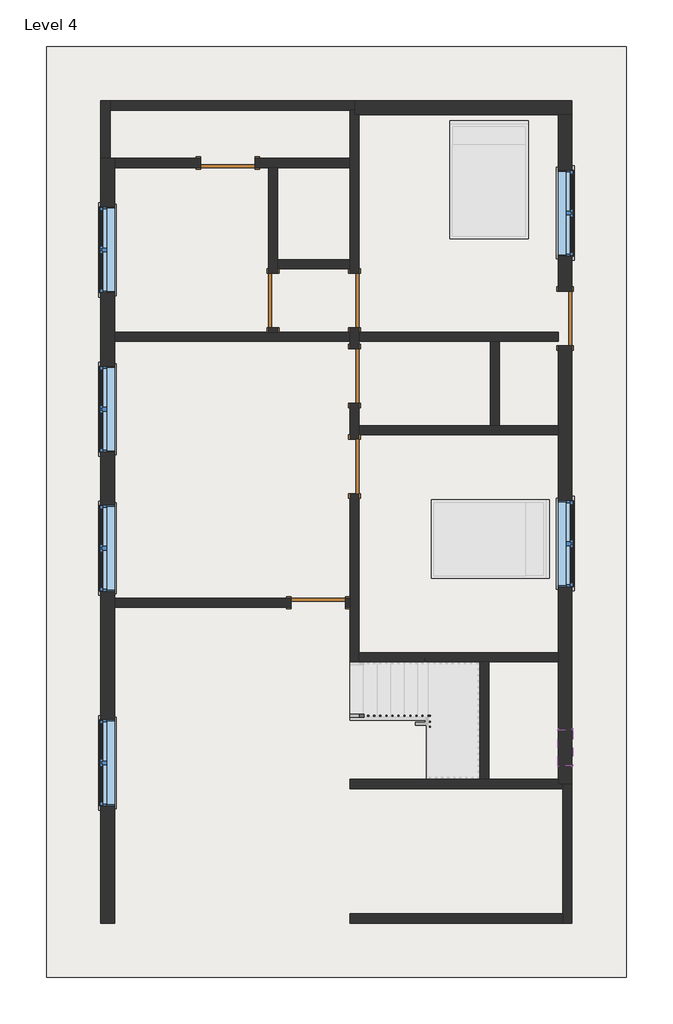
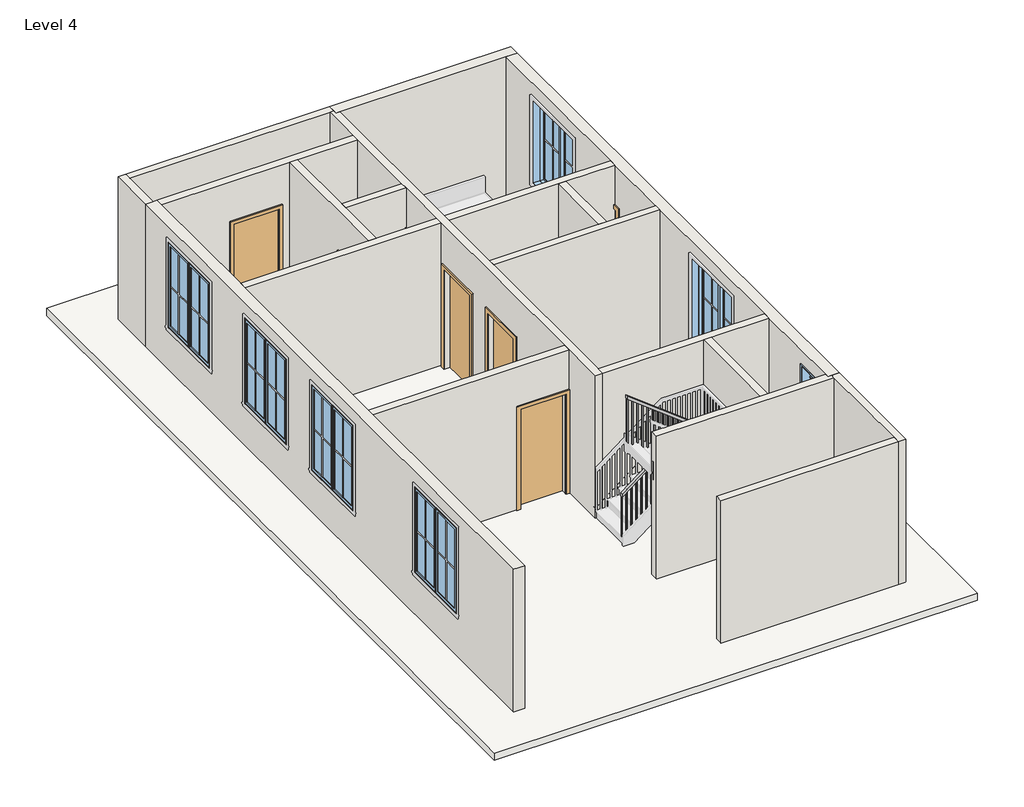
# One storey, part 1 of 2: 18 walls, 7 doors, 7 windows, 1 railing, 1 roof.
"""IFC4 building model written with IfcOpenShell, lengths in millimetres."""

from ifc_helpers import new_model, si_unit, frame, origin, place, context, project, spatial, polyline, outline, extrude, faceted_brep, transform, mapped, element, save
from components import door_686f89d2, door_16372e1c, door_0ca8825f, window_9ac97e1a, window_f2d8fef0

model = new_model("IFC4")

# Units and contexts
model_context = context("Model", 3, world=origin())
ifc_project = project(units=[si_unit("LENGTHUNIT", "METRE", prefix="MILLI")], contexts=[model_context])

# Site, building, storey
site = spatial("IfcSite", under=ifc_project)
building = spatial("IfcBuilding", under=site)
storey = spatial("IfcBuildingStorey", under=building, Name="Level 4", Elevation=6400.8)

# Doors
placement = place(None, origin())
door_shape = door_686f89d2(model_context)
element("IfcDoor", 1, ObjectType="Single-Flush : 36\" x 84\"", at=placement, inside=storey, context=model_context, shape_type="MappedRepresentation", body=[
    mapped(door_shape, transform((-2318.0415352, 3143.9226491, 6400.8), x_axis=(0.0, -1.0, 0.0), y_axis=(1.0, 0.0, 0.0), z_axis=(0.0, 0.0, 1.0))),
])
element("IfcDoor", 2, ObjectType="Single-Flush : 36\" x 84\"", at=placement, inside=storey, context=model_context, shape_type="MappedRepresentation", body=[
    mapped(door_shape, transform((-946.4415352, 3143.7222669, 6400.8), x_axis=(0.0, 1.0, 0.0), y_axis=(-1.0, 0.0, 0.0), z_axis=(0.0, 0.0, 1.0))),
])
element("IfcDoor", 3, ObjectType="Single-Flush : 36\" x 84\"", at=placement, inside=storey, context=model_context, shape_type="MappedRepresentation", body=[
    mapped(door_shape, transform((-946.4415352, 1874.1230313, 6400.8), x_axis=(0.0, 1.0, 0.0), y_axis=(-1.0, 0.0, 0.0), z_axis=(0.0, 0.0, 1.0))),
])
element("IfcDoor", 4, ObjectType="Single-Flush : 36\" x 84\"", at=placement, inside=storey, context=model_context, shape_type="MappedRepresentation", body=[
    mapped(door_shape, transform((-946.4415352, 350.1230313, 6400.8), x_axis=(0.0, 1.0, 0.0), y_axis=(-1.0, 0.0, 0.0), z_axis=(0.0, 0.0, 1.0))),
])
element("IfcDoor", 5, ObjectType="Single-Flush : 36\" x 84\"", at=placement, inside=storey, context=model_context, shape_type="MappedRepresentation", body=[
    mapped(door_shape, transform((-3080.0415352, 5453.9645078, 6400.8), x_axis=(1.0, 0.0, 0.0), y_axis=(0.0, 1.0, 0.0), z_axis=(0.0, 0.0, 1.0))),
])
door_2_shape = door_16372e1c(model_context)
element("IfcDoor", 6, ObjectType="Single-Flush : 36\" x 84\"", at=placement, inside=storey, context=model_context, shape_type="MappedRepresentation", body=[
    mapped(door_2_shape, transform((-1556.0415352, -1935.8769687, 6400.8), x_axis=(1.0, 0.0, 0.0), y_axis=(0.0, 1.0, 0.0), z_axis=(0.0, 0.0, 1.0))),
])
door_3_shape = door_0ca8825f(model_context)
element("IfcDoor", 7, ObjectType="Single-Flush : 36\" x 84\"", at=placement, inside=storey, context=model_context, shape_type="MappedRepresentation", body=[
    mapped(door_3_shape, transform((2596.8584648, 2839.3230313, 6400.8), x_axis=(0.0, -1.0, 0.0), y_axis=(1.0, 0.0, 0.0), z_axis=(0.0, 0.0, 1.0))),
])

# Railing
element("IfcRailing", 8, ObjectType="Handrail - Rectangular", at=placement, inside=storey, context=model_context, shape_type="SolidModel", body=[
    faceted_brep([(-1022.6415352, -3810.4539367, 7484.5333333), (-1022.6415352, -3810.4539367, 7420.3783974), (-1022.6415352, -3861.2539367, 7420.3783974), (-1022.6415352, -3861.2539367, 7484.5333333), (218.4221038, -3810.4539367, 8441.7605883), (269.2221038, -3810.4539367, 8416.7874824), (269.2221038, -3861.2539367, 8416.7874824), (218.4221038, -3861.2539367, 8441.7605883), (218.4221038, -3810.4539367, 8500.5333333), (269.2221038, -3810.4539367, 8449.7333333), (269.2221038, -3861.2539367, 8449.7333333), (218.4221038, -3861.2539367, 8500.5333333), (345.4221038, -3810.4539367, 8500.5333333), (345.4221038, -3810.4539367, 8449.7333333), (294.6221038, -3861.2539367, 8449.7333333), (294.6221038, -3861.2539367, 8500.5333333), (345.4221038, -3937.4539367, 8500.5333333), (345.4221038, -3937.4539367, 8449.7333333), (294.6221038, -3937.4539367, 8449.7333333), (294.6221038, -3937.4539367, 8500.5333333), (345.4221038, -3993.2769687, 8500.5333333), (294.6221038, -3993.2769687, 8500.5333333), (294.6221038, -4044.0769687, 8449.7333333), (345.4221038, -4044.0769687, 8449.7333333)], [[[0, 1, 2, 3]], [[1, 0, 4, 5]], [[2, 1, 5, 6]], [[3, 2, 6, 7]], [[0, 3, 7, 4]], [[5, 4, 8, 9]], [[6, 5, 9, 10]], [[7, 6, 10, 11]], [[4, 7, 11, 8]], [[9, 8, 12, 13]], [[10, 9, 13, 14]], [[11, 10, 14, 15]], [[8, 11, 15, 12]], [[13, 12, 16, 17]], [[14, 13, 17, 18]], [[15, 14, 18, 19]], [[12, 15, 19, 16]], [[20, 21, 22, 23]], [[17, 16, 20, 23]], [[18, 17, 23, 22]], [[19, 18, 22, 21]], [[16, 19, 21, 20]]]),
    faceted_brep([(345.4221038, -3993.2769687, 8500.5333333), (345.4221038, -4044.0769687, 8449.7333333), (294.6221038, -4044.0769687, 8449.7333333), (294.6221038, -3993.2769687, 8500.5333333), (345.4221038, -3993.2769687, 8630.6848366), (294.6221038, -3993.2769687, 8605.7117307), (294.6221038, -4044.0769687, 8605.7117307), (345.4221038, -4044.0769687, 8630.6848366)], [[[0, 1, 2, 3]], [[4, 5, 6, 7]], [[1, 0, 4, 7]], [[2, 1, 7, 6]], [[3, 2, 6, 5]], [[0, 3, 5, 4]]]),
    faceted_brep([(345.4221038, -4044.0769687, 8630.6848366), (294.6221038, -4044.0769687, 8605.7117307), (294.6221038, -3993.2769687, 8605.7117307), (345.4221038, -3993.2769687, 8630.6848366), (-1022.6415352, -4044.0769687, 9685.8666667), (-1022.6415352, -3993.2769687, 9685.8666667), (-1022.6415352, -3993.2769687, 9621.7117307), (-1022.6415352, -4044.0769687, 9621.7117307)], [[[0, 1, 2, 3]], [[4, 5, 6, 7]], [[1, 0, 4, 7]], [[2, 1, 7, 6]], [[3, 2, 6, 5]], [[0, 3, 5, 4]]]),
    extrude(outline(polyline([(9597.5018032, -991.2528962), (9612.1949894, -1010.3028962), (8602.1333333, -1010.3028962), (8602.1333333, -991.2528962), (9597.5018032, -991.2528962)])), frame((0.0, -4028.2019687, 0.0), z_axis=(0.0, 1.0, 0.0), x_axis=(0.0, 0.0, 1.0)), (0.0, 0.0, 1.0), 19.05),
    extrude(outline(polyline([(9519.1381431, -889.6528962), (9533.8313294, -908.7028962), (8602.1333333, -908.7028962), (8602.1333333, -889.6528962), (9519.1381431, -889.6528962)])), frame((0.0, -4028.2019687, 0.0), z_axis=(0.0, 1.0, 0.0), x_axis=(0.0, 0.0, 1.0)), (0.0, 0.0, 1.0), 19.05),
    extrude(outline(polyline([(9440.7744831, -788.0528962), (9455.4676694, -807.1028962), (8602.1333333, -807.1028962), (8602.1333333, -788.0528962), (9440.7744831, -788.0528962)])), frame((0.0, -4028.2019687, 0.0), z_axis=(0.0, 1.0, 0.0), x_axis=(0.0, 0.0, 1.0)), (0.0, 0.0, 1.0), 19.05),
    extrude(outline(polyline([(9362.4108231, -686.4528962), (9377.1040093, -705.5028962), (8432.8, -705.5028962), (8432.8, -686.4528962), (9362.4108231, -686.4528962)])), frame((0.0, -4028.2019687, 0.0), z_axis=(0.0, 1.0, 0.0), x_axis=(0.0, 0.0, 1.0)), (0.0, 0.0, 1.0), 19.05),
    extrude(outline(polyline([(9284.047163, -584.8528962), (9298.7403493, -603.9028962), (8432.8, -603.9028962), (8432.8, -584.8528962), (9284.047163, -584.8528962)])), frame((0.0, -4028.2019687, 0.0), z_axis=(0.0, 1.0, 0.0), x_axis=(0.0, 0.0, 1.0)), (0.0, 0.0, 1.0), 19.05),
    extrude(outline(polyline([(9205.683503, -483.2528962), (9220.3766892, -502.3028962), (8263.4666667, -502.3028962), (8263.4666667, -483.2528962), (9205.683503, -483.2528962)])), frame((0.0, -4028.2019687, 0.0), z_axis=(0.0, 1.0, 0.0), x_axis=(0.0, 0.0, 1.0)), (0.0, 0.0, 1.0), 19.05),
    extrude(outline(polyline([(9127.3198429, -381.6528962), (9142.0130292, -400.7028962), (8263.4666667, -400.7028962), (8263.4666667, -381.6528962), (9127.3198429, -381.6528962)])), frame((0.0, -4028.2019687, 0.0), z_axis=(0.0, 1.0, 0.0), x_axis=(0.0, 0.0, 1.0)), (0.0, 0.0, 1.0), 19.05),
    extrude(outline(polyline([(9048.9561829, -280.0528962), (9063.6493691, -299.1028962), (8094.1333333, -299.1028962), (8094.1333333, -280.0528962), (9048.9561829, -280.0528962)])), frame((0.0, -4028.2019687, 0.0), z_axis=(0.0, 1.0, 0.0), x_axis=(0.0, 0.0, 1.0)), (0.0, 0.0, 1.0), 19.05),
    extrude(outline(polyline([(8970.5925228, -178.4528962), (8985.2857091, -197.5028962), (8094.1333333, -197.5028962), (8094.1333333, -178.4528962), (8970.5925228, -178.4528962)])), frame((0.0, -4028.2019687, 0.0), z_axis=(0.0, 1.0, 0.0), x_axis=(0.0, 0.0, 1.0)), (0.0, 0.0, 1.0), 19.05),
    extrude(outline(polyline([(8892.2288628, -76.8528962), (8906.922049, -95.9028962), (7924.8, -95.9028962), (7924.8, -76.8528962), (8892.2288628, -76.8528962)])), frame((0.0, -4028.2019687, 0.0), z_axis=(0.0, 1.0, 0.0), x_axis=(0.0, 0.0, 1.0)), (0.0, 0.0, 1.0), 19.05),
    extrude(outline(polyline([(8813.8652027, 24.7471038), (8828.558389, 5.6971038), (7924.8, 5.6971038), (7924.8, 24.7471038), (8813.8652027, 24.7471038)])), frame((0.0, -4028.2019687, 0.0), z_axis=(0.0, 1.0, 0.0), x_axis=(0.0, 0.0, 1.0)), (0.0, 0.0, 1.0), 19.05),
    extrude(outline(polyline([(8735.5015427, 126.3471038), (8750.1947289, 107.2971038), (7924.8, 107.2971038), (7924.8, 126.3471038), (8735.5015427, 126.3471038)])), frame((0.0, -4028.2019687, 0.0), z_axis=(0.0, 1.0, 0.0), x_axis=(0.0, 0.0, 1.0)), (0.0, 0.0, 1.0), 19.05),
    extrude(outline(polyline([(8657.1378826, 227.9471038), (8671.8310689, 208.8971038), (7755.4666667, 208.8971038), (7755.4666667, 227.9471038), (8657.1378826, 227.9471038)])), frame((0.0, -4028.2019687, 0.0), z_axis=(0.0, 1.0, 0.0), x_axis=(0.0, 0.0, 1.0)), (0.0, 0.0, 1.0), 19.05),
    extrude(outline(polyline([(310.4971038, -3927.9289367), (329.5471038, -3927.9289367), (329.5471038, -3946.9789367), (310.4971038, -3946.9789367), (310.4971038, -3927.9289367)])), frame((0.0, 0.0, 7586.1333333), z_axis=(0.0, 0.0, 1.0), x_axis=(1.0, 0.0, 0.0)), (0.0, 0.0, 1.0), 863.6),
    extrude(outline(polyline([(288.6334648, -3845.3789367), (288.6334648, -3826.3289367), (307.6834648, -3826.3289367), (307.6834648, -3845.3789367), (288.6334648, -3845.3789367)])), frame((0.0, 0.0, 7586.1333333), z_axis=(0.0, 0.0, 1.0), x_axis=(1.0, 0.0, 0.0)), (0.0, 0.0, 1.0), 863.6),
    extrude(outline(polyline([(8368.0889111, 206.0834648), (8353.3957248, 187.0334648), (7416.8, 187.0334648), (7416.8, 206.0834648), (8368.0889111, 206.0834648)])), frame((0.0, -3845.3789367, 0.0), z_axis=(0.0, 1.0, 0.0), x_axis=(0.0, 0.0, 1.0)), (0.0, 0.0, 1.0), 19.05),
    extrude(outline(polyline([(8289.725251, 104.4834648), (8275.0320648, 85.4334648), (7247.4666667, 85.4334648), (7247.4666667, 104.4834648), (8289.725251, 104.4834648)])), frame((0.0, -3845.3789367, 0.0), z_axis=(0.0, 1.0, 0.0), x_axis=(0.0, 0.0, 1.0)), (0.0, 0.0, 1.0), 19.05),
    extrude(outline(polyline([(8211.361591, 2.8834648), (8196.6684047, -16.1665352), (7247.4666667, -16.1665352), (7247.4666667, 2.8834648), (8211.361591, 2.8834648)])), frame((0.0, -3845.3789367, 0.0), z_axis=(0.0, 1.0, 0.0), x_axis=(0.0, 0.0, 1.0)), (0.0, 0.0, 1.0), 19.05),
    extrude(outline(polyline([(8132.9979309, -98.7165352), (8118.3047447, -117.7665352), (7247.4666667, -117.7665352), (7247.4666667, -98.7165352), (8132.9979309, -98.7165352)])), frame((0.0, -3845.3789367, 0.0), z_axis=(0.0, 1.0, 0.0), x_axis=(0.0, 0.0, 1.0)), (0.0, 0.0, 1.0), 19.05),
    extrude(outline(polyline([(8054.6342709, -200.3165352), (8039.9410846, -219.3665352), (7078.1333333, -219.3665352), (7078.1333333, -200.3165352), (8054.6342709, -200.3165352)])), frame((0.0, -3845.3789367, 0.0), z_axis=(0.0, 1.0, 0.0), x_axis=(0.0, 0.0, 1.0)), (0.0, 0.0, 1.0), 19.05),
    extrude(outline(polyline([(7976.2706109, -301.9165352), (7961.5774246, -320.9665352), (7078.1333333, -320.9665352), (7078.1333333, -301.9165352), (7976.2706109, -301.9165352)])), frame((0.0, -3845.3789367, 0.0), z_axis=(0.0, 1.0, 0.0), x_axis=(0.0, 0.0, 1.0)), (0.0, 0.0, 1.0), 19.05),
    extrude(outline(polyline([(7897.9069508, -403.5165352), (7883.2137645, -422.5665352), (6908.8, -422.5665352), (6908.8, -403.5165352), (7897.9069508, -403.5165352)])), frame((0.0, -3845.3789367, 0.0), z_axis=(0.0, 1.0, 0.0), x_axis=(0.0, 0.0, 1.0)), (0.0, 0.0, 1.0), 19.05),
    extrude(outline(polyline([(7819.5432908, -505.1165352), (7804.8501045, -524.1665352), (6908.8, -524.1665352), (6908.8, -505.1165352), (7819.5432908, -505.1165352)])), frame((0.0, -3845.3789367, 0.0), z_axis=(0.0, 1.0, 0.0), x_axis=(0.0, 0.0, 1.0)), (0.0, 0.0, 1.0), 19.05),
    extrude(outline(polyline([(7741.1796307, -606.7165352), (7726.4864445, -625.7665352), (6739.4666667, -625.7665352), (6739.4666667, -606.7165352), (7741.1796307, -606.7165352)])), frame((0.0, -3845.3789367, 0.0), z_axis=(0.0, 1.0, 0.0), x_axis=(0.0, 0.0, 1.0)), (0.0, 0.0, 1.0), 19.05),
    extrude(outline(polyline([(7662.8159707, -708.3165352), (7648.1227844, -727.3665352), (6739.4666667, -727.3665352), (6739.4666667, -708.3165352), (7662.8159707, -708.3165352)])), frame((0.0, -3845.3789367, 0.0), z_axis=(0.0, 1.0, 0.0), x_axis=(0.0, 0.0, 1.0)), (0.0, 0.0, 1.0), 19.05),
    extrude(outline(polyline([(7584.4523106, -809.9165352), (7569.7591244, -828.9665352), (6570.1333333, -828.9665352), (6570.1333333, -809.9165352), (7584.4523106, -809.9165352)])), frame((0.0, -3845.3789367, 0.0), z_axis=(0.0, 1.0, 0.0), x_axis=(0.0, 0.0, 1.0)), (0.0, 0.0, 1.0), 19.05),
    extrude(outline(polyline([(7506.0886506, -911.5165352), (7491.3954643, -930.5665352), (6570.1333333, -930.5665352), (6570.1333333, -911.5165352), (7506.0886506, -911.5165352)])), frame((0.0, -3845.3789367, 0.0), z_axis=(0.0, 1.0, 0.0), x_axis=(0.0, 0.0, 1.0)), (0.0, 0.0, 1.0), 19.05),
    extrude(outline(polyline([(310.4971038, -4009.1519687), (329.5471038, -4009.1519687), (329.5471038, -4028.2019687), (310.4971038, -4028.2019687), (310.4971038, -4009.1519687)])), frame((0.0, 0.0, 7586.1333333), z_axis=(0.0, 0.0, 1.0), x_axis=(1.0, 0.0, 0.0)), (0.0, 0.0, 1.0), 863.6),
    extrude(outline(polyline([(310.4971038, -3845.3789367), (310.4971038, -3826.3289367), (329.5471038, -3826.3289367), (329.5471038, -3845.3789367), (310.4971038, -3845.3789367)])), frame((0.0, 0.0, 7586.1333333), z_axis=(0.0, 0.0, 1.0), x_axis=(1.0, 0.0, 0.0)), (0.0, 0.0, 1.0), 863.6),
    extrude(outline(polyline([(9607.0185445, -1003.5915352), (9621.7117307, -1022.6415352), (8602.1333333, -1022.6415352), (8602.1333333, -1003.5915352), (9607.0185445, -1003.5915352)])), frame((0.0, -4028.2019687, 0.0), z_axis=(0.0, 1.0, 0.0), x_axis=(0.0, 0.0, 1.0)), (0.0, 0.0, 1.0), 19.05),
    extrude(outline(polyline([(7435.0715837, -1003.5915352), (7420.3783974, -1022.6415352), (6570.1333333, -1022.6415352), (6570.1333333, -1003.5915352), (7435.0715837, -1003.5915352)])), frame((0.0, -3845.3789367, 0.0), z_axis=(0.0, 1.0, 0.0), x_axis=(0.0, 0.0, 1.0)), (0.0, 0.0, 1.0), 19.05),
])

# Roof
element("IfcRoof", 9, ObjectType="ROOF 6\"", at=placement, inside=storey, context=model_context, shape_type="SweptSolid", body=[
    extrude(outline(polyline([(-6128.0415352, 7411.3230313), (3625.5584648, 7411.3230313), (3625.5584648, -8235.0769687), (-6128.0415352, -8235.0769687), (-6128.0415352, 7411.3230313)])), frame((0.0, 0.0, 6248.4), z_axis=(0.0, 0.0, 1.0), x_axis=(1.0, 0.0, 0.0)), (0.0, 0.0, 1.0), 152.4),
])

# Walls
element("IfcWall", 10, ObjectType="WALL 6\"", at=placement, inside=storey, context=model_context, shape_type="Brep", body=[
    faceted_brep([(-5061.2415352, 5531.7230313, 6400.8), (-5061.2415352, 6344.5230313, 6400.8), (-5061.2415352, 6496.9230313, 6400.8), (-5061.2415352, 6496.9230313, 9448.8), (-5061.2415352, 6344.5230313, 9448.8), (-5061.2415352, 5531.7230313, 9448.8), (-5213.6415352, 5531.7230313, 6400.8), (-5213.6415352, 5531.7230313, 9448.8), (-5213.6415352, 6496.9230313, 9448.8), (-5213.6415352, 6496.9230313, 6400.8)], [[[0, 1, 2, 3, 4, 5]], [[6, 7, 8, 9]], [[2, 1, 0, 6, 9]], [[0, 5, 7, 6]], [[3, 2, 9, 8]], [[5, 4, 3, 8, 7]]]),
])
element("IfcWall", 11, ObjectType="WALL 6\"", at=placement, inside=storey, context=model_context, shape_type="Brep", body=[
    faceted_brep([(-5061.2415352, 6344.5230313, 6400.8), (-1022.6415352, 6344.5230313, 6400.8), (-946.4415352, 6344.5230313, 6400.8), (-946.4415352, 6344.5230313, 9448.8), (-1022.6415352, 6344.5230313, 9448.8), (-5061.2415352, 6344.5230313, 9448.8), (-5061.2415352, 6496.9230313, 6400.8), (-5061.2415352, 6496.9230313, 9448.8), (-946.4415352, 6496.9230313, 9448.8), (-946.4415352, 6496.9230313, 6400.8)], [[[0, 1, 2, 3, 4, 5]], [[6, 7, 8, 9]], [[2, 1, 0, 6, 9]], [[3, 2, 9, 8]], [[0, 5, 7, 6]], [[5, 4, 3, 8, 7]]]),
])
element("IfcWall", 12, ObjectType="WALL 6\"", at=placement, inside=storey, context=model_context, shape_type="Brep", body=[
    faceted_brep([(-1022.6415352, 1416.9230313, 6400.8), (-1022.6415352, 807.3230313, 6400.8), (-1022.6415352, 807.3230313, 8534.4), (-1022.6415352, -107.0769687, 8534.4), (-1022.6415352, -107.0769687, 6400.8), (-1022.6415352, -1859.6769687, 6400.8), (-1022.6415352, -2012.0769687, 6400.8), (-1022.6415352, -2926.4769687, 6400.8), (-1022.6415352, -2926.4769687, 9448.8), (-1022.6415352, -2012.0769687, 9448.8), (-1022.6415352, -1859.6769687, 9448.8), (-1022.6415352, 2458.3230313, 9448.8), (-1022.6415352, 2610.7230313, 9448.8), (-1022.6415352, 3677.1222669, 9448.8), (-1022.6415352, 3829.5222669, 9448.8), (-1022.6415352, 5377.7645078, 9448.8), (-1022.6415352, 5530.1645078, 9448.8), (-1022.6415352, 6344.5230313, 9448.8), (-1022.6415352, 6344.5230313, 6400.8), (-1022.6415352, 5530.1645078, 6400.8), (-1022.6415352, 5377.7645078, 6400.8), (-1022.6415352, 3829.5222669, 6400.8), (-1022.6415352, 3677.1222669, 6400.8), (-1022.6415352, 3600.9222669, 6400.8), (-1022.6415352, 3600.9222669, 8534.4), (-1022.6415352, 2686.5222669, 8534.4), (-1022.6415352, 2686.5222669, 6400.8), (-1022.6415352, 2610.7230313, 6400.8), (-1022.6415352, 2458.3230313, 6400.8), (-1022.6415352, 2331.3230313, 6400.8), (-1022.6415352, 2331.3230313, 8534.4), (-1022.6415352, 1416.9230313, 8534.4), (-870.2415352, 807.3230313, 8534.4), (-870.2415352, 807.3230313, 6400.8), (-870.2415352, 883.5230313, 6400.8), (-870.2415352, 1035.9230313, 6400.8), (-870.2415352, 1416.9230313, 6400.8), (-870.2415352, 1416.9230313, 8534.4), (-870.2415352, 2331.3230313, 8534.4), (-870.2415352, 2331.3230313, 6400.8), (-870.2415352, 2458.3230313, 6400.8), (-870.2415352, 2610.7230313, 6400.8), (-870.2415352, 2686.5222669, 6400.8), (-870.2415352, 2686.5222669, 8534.4), (-870.2415352, 3600.9222669, 8534.4), (-870.2415352, 3600.9222669, 6400.8), (-870.2415352, 6268.3230313, 6400.8), (-870.2415352, 6268.3230313, 9448.8), (-870.2415352, 2610.7230313, 9448.8), (-870.2415352, 2458.3230313, 9448.8), (-870.2415352, 1035.9230313, 9448.8), (-870.2415352, 883.5230313, 9448.8), (-870.2415352, -2774.0769687, 9448.8), (-870.2415352, -2926.4769687, 9448.8), (-870.2415352, -2926.4769687, 6400.8), (-870.2415352, -2774.0769687, 6400.8), (-870.2415352, -107.0769687, 6400.8), (-870.2415352, -107.0769687, 8534.4), (-946.4415352, 6344.5230313, 6400.8), (-946.4415352, 6268.3230313, 6400.8), (-946.4415352, 6344.5230313, 9448.8), (-946.4415352, 6268.3230313, 9448.8)], [[[0, 1, 2, 3, 4, 5, 6, 7, 8, 9, 10, 11, 12, 13, 14, 15, 16, 17, 18, 19, 20, 21, 22, 23, 24, 25, 26, 27, 28, 29, 30, 31]], [[32, 33, 34, 35, 36, 37, 38, 39, 40, 41, 42, 43, 44, 45, 46, 47, 48, 49, 50, 51, 52, 53, 54, 55, 56, 57]], [[46, 45, 23, 22, 21, 20, 19, 18, 58, 59]], [[42, 41, 40, 39, 29, 28, 27, 26]], [[56, 55, 54, 7, 6, 5, 4]], [[36, 35, 34, 33, 1, 0]], [[18, 17, 60, 58]], [[60, 61, 59, 58]], [[61, 47, 46, 59]], [[8, 7, 54, 53]], [[24, 23, 45, 44]], [[25, 24, 44, 43]], [[26, 25, 43, 42]], [[30, 29, 39, 38]], [[31, 30, 38, 37]], [[0, 31, 37, 36]], [[2, 1, 33, 32]], [[3, 2, 32, 57]], [[4, 3, 57, 56]], [[17, 16, 15, 14, 13, 12, 11, 10, 9, 8, 53, 52, 51, 50, 49, 48, 47, 61, 60]]]),
])
element("IfcWall", 13, ObjectType="WALL 6\"", at=placement, inside=storey, context=model_context, shape_type="Brep", body=[
    faceted_brep([(2482.5584648, -2774.0769687, 6400.8), (-870.2415352, -2774.0769687, 6400.8), (-870.2415352, -2774.0769687, 9448.8), (2482.5584648, -2774.0769687, 9448.8), (2482.5584648, -2926.4769687, 6400.8), (2482.5584648, -2926.4769687, 9448.8), (1314.1584648, -2926.4769687, 9448.8), (1161.7584648, -2926.4769687, 9448.8), (-870.2415352, -2926.4769687, 9448.8), (-870.2415352, -2926.4769687, 6400.8), (1161.7584648, -2926.4769687, 6400.8), (1314.1584648, -2926.4769687, 6400.8)], [[[0, 1, 2, 3]], [[4, 5, 6, 7, 8, 9, 10, 11]], [[1, 0, 4, 11, 10, 9]], [[2, 1, 9, 8]], [[0, 3, 5, 4]], [[3, 2, 8, 7, 6, 5]]]),
])
element("IfcWall", 14, ObjectType="WALL 6\"", at=placement, inside=storey, context=model_context, shape_type="Brep", body=[
    faceted_brep([(2558.7584648, -4983.8769687, 6400.8), (2558.7584648, -5060.0769687, 6400.8), (2558.7584648, -7168.2769687, 6400.8), (2558.7584648, -7320.6769687, 6400.8), (2558.7584648, -7320.6769687, 9448.8), (2558.7584648, -7168.2769687, 9448.8), (2558.7584648, -5060.0769687, 9448.8), (2558.7584648, -4983.8769687, 9448.8), (2711.1584648, -4983.8769687, 6400.8), (2711.1584648, -4983.8769687, 9448.8), (2711.1584648, -7320.6769687, 9448.8), (2711.1584648, -7320.6769687, 6400.8)], [[[0, 1, 2, 3, 4, 5, 6, 7]], [[8, 9, 10, 11]], [[3, 2, 1, 0, 8, 11]], [[0, 7, 9, 8]], [[4, 3, 11, 10]], [[7, 6, 5, 4, 10, 9]]]),
])
element("IfcWall", 15, ObjectType="WALL 6\"", at=placement, inside=storey, context=model_context, shape_type="SweptSolid", body=[
    extrude(outline(polyline([(-1022.6415352, -7168.2769687), (2558.7584648, -7168.2769687), (2558.7584648, -7320.6769687), (-1022.6415352, -7320.6769687), (-1022.6415352, -7168.2769687)])), frame((0.0, 0.0, 6400.8), z_axis=(0.0, 0.0, 1.0), x_axis=(1.0, 0.0, 0.0)), (0.0, 0.0, 1.0), 3048.0),
])
element("IfcWall", 16, ObjectType="WALL 6\"", at=placement, inside=storey, context=model_context, shape_type="Brep", body=[
    faceted_brep([(2482.5584648, -4907.6769687, 6400.8), (1314.1584648, -4907.6769687, 6400.8), (1161.7584648, -4907.6769687, 6400.8), (-1022.6415352, -4907.6769687, 6400.8), (-1022.6415352, -4907.6769687, 9448.8), (1161.7584648, -4907.6769687, 9448.8), (1314.1584648, -4907.6769687, 9448.8), (2482.5584648, -4907.6769687, 9448.8), (2558.7584648, -5060.0769687, 6400.8), (2558.7584648, -5060.0769687, 9448.8), (-1022.6415352, -5060.0769687, 9448.8), (-1022.6415352, -5060.0769687, 6400.8), (2482.5584648, -4983.8769687, 6400.8), (2558.7584648, -4983.8769687, 6400.8), (2482.5584648, -4983.8769687, 9448.8), (2558.7584648, -4983.8769687, 9448.8)], [[[0, 1, 2, 3, 4, 5, 6, 7]], [[8, 9, 10, 11]], [[3, 2, 1, 0, 12, 13, 8, 11]], [[4, 3, 11, 10]], [[0, 7, 14, 12]], [[14, 15, 13, 12]], [[15, 9, 8, 13]], [[7, 6, 5, 4, 10, 9, 15, 14]]]),
])
element("IfcWall", 17, ObjectType="WALL 6\"", at=placement, inside=storey, context=model_context, shape_type="SweptSolid", body=[
    extrude(outline(polyline([(1161.7584648, -4907.6769687), (1161.7584648, -2926.4769687), (1314.1584648, -2926.4769687), (1314.1584648, -4907.6769687), (1161.7584648, -4907.6769687)])), frame((0.0, 0.0, 6400.8), z_axis=(0.0, 0.0, 1.0), x_axis=(1.0, 0.0, 0.0)), (0.0, 0.0, 1.0), 3048.0),
])
element("IfcWall", 18, ObjectType="WALL 6\"", at=placement, inside=storey, context=model_context, shape_type="SweptSolid", body=[
    extrude(outline(polyline([(8534.4, -1098.8415352), (6400.8, -1098.8415352), (6400.8, -1022.6415352), (9448.8, -1022.6415352), (9448.8, -4985.0415352), (6400.8, -4985.0415352), (6400.8, -2013.2415352), (8534.4, -2013.2415352), (8534.4, -1098.8415352)])), frame((0.0, -2012.0769687, 0.0), z_axis=(0.0, 1.0, 0.0), x_axis=(0.0, 0.0, 1.0)), (0.0, 0.0, 1.0), 152.4),
])
element("IfcWall", 19, ObjectType="WALL 6\"", at=placement, inside=storey, context=model_context, shape_type="Brep", body=[
    faceted_brep([(2482.5584648, 2458.3230313, 6400.8), (2482.5584648, 2458.3230313, 9448.8), (1491.9584648, 2458.3230313, 9448.8), (1339.5584648, 2458.3230313, 9448.8), (-870.2415352, 2458.3230313, 9448.8), (-870.2415352, 2458.3230313, 6400.8), (1339.5584648, 2458.3230313, 6400.8), (1491.9584648, 2458.3230313, 6400.8), (2482.5584648, 2610.7230313, 9448.8), (2482.5584648, 2610.7230313, 6400.8), (-870.2415352, 2610.7230313, 6400.8), (-870.2415352, 2610.7230313, 9448.8)], [[[0, 1, 2, 3, 4, 5, 6, 7]], [[8, 9, 10, 11]], [[9, 0, 7, 6, 5, 10]], [[1, 0, 9, 8]], [[5, 4, 11, 10]], [[1, 8, 11, 4, 3, 2]]]),
    faceted_brep([(-4985.0415352, 2458.3230313, 9448.8), (-4985.0415352, 2458.3230313, 6400.8), (-1022.6415352, 2458.3230313, 6400.8), (-1022.6415352, 2458.3230313, 9448.8), (-4985.0415352, 2610.7230313, 6400.8), (-4985.0415352, 2610.7230313, 9448.8), (-2394.2415352, 2610.7230313, 9448.8), (-2241.8415352, 2610.7230313, 9448.8), (-1022.6415352, 2610.7230313, 9448.8), (-1022.6415352, 2610.7230313, 6400.8), (-2241.8415352, 2610.7230313, 6400.8), (-2394.2415352, 2610.7230313, 6400.8)], [[[0, 1, 2, 3]], [[4, 5, 6, 7, 8, 9, 10, 11]], [[1, 4, 11, 10, 9, 2]], [[1, 0, 5, 4]], [[3, 2, 9, 8]], [[5, 0, 3, 8, 7, 6]]]),
])
element("IfcWall", 20, ObjectType="WALL 6\"", at=placement, inside=storey, context=model_context, shape_type="Brep", body=[
    faceted_brep([(-2622.8415352, 5377.7645078, 8534.4), (-2622.8415352, 5377.7645078, 6400.8), (-2394.2415352, 5377.7645078, 6400.8), (-2241.8415352, 5377.7645078, 6400.8), (-1022.6415352, 5377.7645078, 6400.8), (-1022.6415352, 5377.7645078, 9448.8), (-2241.8415352, 5377.7645078, 9448.8), (-2394.2415352, 5377.7645078, 9448.8), (-4985.0415352, 5377.7645078, 9448.8), (-4985.0415352, 5377.7645078, 6400.8), (-3537.2415352, 5377.7645078, 6400.8), (-3537.2415352, 5377.7645078, 8534.4), (-1022.6415352, 5530.1645078, 6400.8), (-2622.8415352, 5530.1645078, 6400.8), (-2622.8415352, 5530.1645078, 8534.4), (-3537.2415352, 5530.1645078, 8534.4), (-3537.2415352, 5530.1645078, 6400.8), (-4985.0415352, 5530.1645078, 6400.8), (-4985.0415352, 5530.1645078, 9448.8), (-1022.6415352, 5530.1645078, 9448.8)], [[[0, 1, 2, 3, 4, 5, 6, 7, 8, 9, 10, 11]], [[12, 13, 14, 15, 16, 17, 18, 19]], [[10, 9, 17, 16]], [[4, 3, 2, 1, 13, 12]], [[9, 8, 18, 17]], [[5, 4, 12, 19]], [[14, 13, 1, 0]], [[15, 14, 0, 11]], [[16, 15, 11, 10]], [[8, 7, 6, 5, 19, 18]]]),
])
element("IfcWall", 21, ObjectType="WALL 6\"", at=placement, inside=storey, context=model_context, shape_type="Brep", body=[
    faceted_brep([(-2394.2415352, 2686.7226491, 8534.4), (-2394.2415352, 2686.7226491, 6400.8), (-2394.2415352, 2610.7230313, 6400.8), (-2394.2415352, 2610.7230313, 9448.8), (-2394.2415352, 5377.7645078, 9448.8), (-2394.2415352, 5377.7645078, 6400.8), (-2394.2415352, 3601.1226491, 6400.8), (-2394.2415352, 3601.1226491, 8534.4), (-2241.8415352, 2610.7230313, 6400.8), (-2241.8415352, 2686.7226491, 6400.8), (-2241.8415352, 2686.7226491, 8534.4), (-2241.8415352, 3601.1226491, 8534.4), (-2241.8415352, 3601.1226491, 6400.8), (-2241.8415352, 3677.1222669, 6400.8), (-2241.8415352, 3829.5222669, 6400.8), (-2241.8415352, 5377.7645078, 6400.8), (-2241.8415352, 5377.7645078, 9448.8), (-2241.8415352, 3829.5222669, 9448.8), (-2241.8415352, 3677.1222669, 9448.8), (-2241.8415352, 2610.7230313, 9448.8)], [[[0, 1, 2, 3, 4, 5, 6, 7]], [[8, 9, 10, 11, 12, 13, 14, 15, 16, 17, 18, 19]], [[6, 5, 15, 14, 13, 12]], [[2, 1, 9, 8]], [[3, 2, 8, 19]], [[5, 4, 16, 15]], [[10, 9, 1, 0]], [[11, 10, 0, 7]], [[12, 11, 7, 6]], [[4, 3, 19, 18, 17, 16]]]),
])
element("IfcWall", 22, ObjectType="WALL 6\"", at=placement, inside=storey, context=model_context, shape_type="SweptSolid", body=[
    extrude(outline(polyline([(-1022.6415352, 3677.1222669), (-2241.8415352, 3677.1222669), (-2241.8415352, 3829.5222669), (-1022.6415352, 3829.5222669), (-1022.6415352, 3677.1222669)])), frame((0.0, 0.0, 6400.8), z_axis=(0.0, 0.0, 1.0), x_axis=(1.0, 0.0, 0.0)), (0.0, 0.0, 1.0), 3048.0),
])
element("IfcWall", 23, ObjectType="WALL 6\"", at=placement, inside=storey, context=model_context, shape_type="Brep", body=[
    faceted_brep([(-870.2415352, 883.5230313, 6400.8), (2482.5584648, 883.5230313, 6400.8), (2482.5584648, 883.5230313, 9448.8), (-870.2415352, 883.5230313, 9448.8), (-870.2415352, 1035.9230313, 6400.8), (-870.2415352, 1035.9230313, 9448.8), (1339.5584648, 1035.9230313, 9448.8), (1491.9584648, 1035.9230313, 9448.8), (2482.5584648, 1035.9230313, 9448.8), (2482.5584648, 1035.9230313, 6400.8), (1491.9584648, 1035.9230313, 6400.8), (1339.5584648, 1035.9230313, 6400.8)], [[[0, 1, 2, 3]], [[4, 5, 6, 7, 8, 9, 10, 11]], [[1, 0, 4, 11, 10, 9]], [[2, 1, 9, 8]], [[0, 3, 5, 4]], [[3, 2, 8, 7, 6, 5]]]),
])
element("IfcWall", 24, ObjectType="WALL 6\"", at=placement, inside=storey, context=model_context, shape_type="SweptSolid", body=[
    extrude(outline(polyline([(1339.5584648, 1035.9230313), (1339.5584648, 2458.3230313), (1491.9584648, 2458.3230313), (1491.9584648, 1035.9230313), (1339.5584648, 1035.9230313)])), frame((0.0, 0.0, 6400.8), z_axis=(0.0, 0.0, 1.0), x_axis=(1.0, 0.0, 0.0)), (0.0, 0.0, 1.0), 3048.0),
])
element("IfcWall", 25, ObjectType="WALL 9\"", at=placement, inside=storey, context=model_context, shape_type="Brep", body=[
    faceted_brep([(-946.4415352, 6268.3230313, 6400.8), (-870.2415352, 6268.3230313, 6400.8), (2482.5584648, 6268.3230313, 6400.8), (2711.1584648, 6268.3230313, 6400.8), (2711.1584648, 6268.3230313, 9448.8), (2482.5584648, 6268.3230313, 9448.8), (-870.2415352, 6268.3230313, 9448.8), (-946.4415352, 6268.3230313, 9448.8), (-946.4415352, 6496.9230313, 6400.8), (-946.4415352, 6496.9230313, 9448.8), (2711.1584648, 6496.9230313, 9448.8), (2711.1584648, 6496.9230313, 6400.8), (-946.4415352, 6344.5230313, 6400.8), (-946.4415352, 6344.5230313, 9448.8)], [[[0, 1, 2, 3, 4, 5, 6, 7]], [[8, 9, 10, 11]], [[3, 2, 1, 0, 12, 8, 11]], [[0, 7, 13, 9, 8, 12]], [[4, 3, 11, 10]], [[7, 6, 5, 4, 10, 9, 13]]]),
])
element("IfcWall", 26, ObjectType="WALL 9\"", at=placement, inside=storey, context=model_context, shape_type="Brep", body=[
    faceted_brep([(2482.5584648, 2382.1230313, 8534.4), (2482.5584648, 2382.1230313, 6400.8), (2482.5584648, 1035.9230313, 6400.8), (2482.5584648, 883.5230313, 6400.8), (2482.5584648, -2774.0769687, 6400.8), (2482.5584648, -2926.4769687, 6400.8), (2482.5584648, -4907.6769687, 6400.8), (2482.5584648, -4983.8769687, 6400.8), (2482.5584648, -4983.8769687, 9448.8), (2482.5584648, -4907.6769687, 9448.8), (2482.5584648, -2926.4769687, 9448.8), (2482.5584648, -2774.0769687, 9448.8), (2482.5584648, 883.5230313, 9448.8), (2482.5584648, 1035.9230313, 9448.8), (2482.5584648, 2458.3230313, 9448.8), (2482.5584648, 2610.7230313, 9448.8), (2482.5584648, 6268.3230313, 9448.8), (2482.5584648, 6268.3230313, 6400.8), (2482.5584648, 3296.5230313, 6400.8), (2482.5584648, 3296.5230313, 8534.4), (2482.5584648, 3887.0730313, 9144.0), (2482.5584648, 3887.0730313, 7315.2), (2482.5584648, 5334.8730313, 7315.2), (2482.5584648, 5334.8730313, 9144.0), (2482.5584648, -1669.1769687, 9144.0), (2482.5584648, -1669.1769687, 7315.2), (2482.5584648, -221.3769687, 7315.2), (2482.5584648, -221.3769687, 9144.0), (2482.5584648, -4069.4769687, 9144.0), (2482.5584648, -4679.0769687, 9144.0), (2482.5584648, -4679.0769687, 8534.4), (2482.5584648, -4069.4769687, 8534.4), (2711.1584648, -4983.8769687, 6400.8), (2711.1584648, 2382.1230313, 6400.8), (2711.1584648, 2382.1230313, 8534.4), (2711.1584648, 3296.5230313, 8534.4), (2711.1584648, 3296.5230313, 6400.8), (2711.1584648, 6268.3230313, 6400.8), (2711.1584648, 6268.3230313, 9448.8), (2711.1584648, -4983.8769687, 9448.8), (2711.1584648, 3887.0730313, 9144.0), (2711.1584648, 5334.8730313, 9144.0), (2711.1584648, 5334.8730313, 7315.2), (2711.1584648, 3887.0730313, 7315.2), (2711.1584648, -1669.1769687, 9144.0), (2711.1584648, -221.3769687, 9144.0), (2711.1584648, -221.3769687, 7315.2), (2711.1584648, -1669.1769687, 7315.2), (2711.1584648, -4069.4769687, 9144.0), (2711.1584648, -4069.4769687, 8534.4), (2711.1584648, -4679.0769687, 8534.4), (2711.1584648, -4679.0769687, 9144.0), (2558.7584648, -4983.8769687, 6400.8), (2558.7584648, -4983.8769687, 9448.8)], [[[0, 1, 2, 3, 4, 5, 6, 7, 8, 9, 10, 11, 12, 13, 14, 15, 16, 17, 18, 19], [20, 21, 22, 23], [24, 25, 26, 27], [28, 29, 30, 31]], [[32, 33, 34, 35, 36, 37, 38, 39], [40, 41, 42, 43], [44, 45, 46, 47], [48, 49, 50, 51]], [[18, 17, 37, 36]], [[7, 6, 5, 4, 3, 2, 1, 33, 32, 52]], [[8, 7, 52, 32, 39, 53]], [[17, 16, 38, 37]], [[34, 33, 1, 0]], [[35, 34, 0, 19]], [[36, 35, 19, 18]], [[21, 20, 40, 43]], [[22, 21, 43, 42]], [[23, 22, 42, 41]], [[20, 23, 41, 40]], [[25, 24, 44, 47]], [[26, 25, 47, 46]], [[27, 26, 46, 45]], [[24, 27, 45, 44]], [[49, 48, 28, 31]], [[50, 49, 31, 30]], [[51, 50, 30, 29]], [[48, 51, 29, 28]], [[16, 15, 14, 13, 12, 11, 10, 9, 8, 53, 39, 38]]]),
])
element("IfcWall", 27, ObjectType="WALL 9\"", at=placement, inside=storey, context=model_context, shape_type="Brep", body=[
    faceted_brep([(-4985.0415352, -7320.6769687, 6400.8), (-4985.0415352, -2012.0769687, 6400.8), (-4985.0415352, -1859.6769687, 6400.8), (-4985.0415352, 2458.3230313, 6400.8), (-4985.0415352, 2610.7230313, 6400.8), (-4985.0415352, 5377.7645078, 6400.8), (-4985.0415352, 5530.1645078, 6400.8), (-4985.0415352, 5531.7230313, 6400.8), (-4985.0415352, 5531.7230313, 9448.8), (-4985.0415352, 5530.1645078, 9448.8), (-4985.0415352, 5377.7645078, 9448.8), (-4985.0415352, 2610.7230313, 9448.8), (-4985.0415352, 2458.3230313, 9448.8), (-4985.0415352, -1859.6769687, 9448.8), (-4985.0415352, -2012.0769687, 9448.8), (-4985.0415352, -7320.6769687, 9448.8), (-4985.0415352, 4718.1437696, 9144.0), (-4985.0415352, 4718.1437696, 7315.2), (-4985.0415352, 3270.3437696, 7315.2), (-4985.0415352, 3270.3437696, 9144.0), (-4985.0415352, 2039.2230313, 9144.0), (-4985.0415352, 2039.2230313, 7315.2), (-4985.0415352, 591.4230313, 7315.2), (-4985.0415352, 591.4230313, 9144.0), (-4985.0415352, -297.5769687, 9144.0), (-4985.0415352, -297.5769687, 7315.2), (-4985.0415352, -1745.3769687, 7315.2), (-4985.0415352, -1745.3769687, 9144.0), (-4985.0415352, -3904.3769687, 9144.0), (-4985.0415352, -3904.3769687, 7315.2), (-4985.0415352, -5352.1769687, 7315.2), (-4985.0415352, -5352.1769687, 9144.0), (-5213.6415352, -7320.6769687, 6400.8), (-5213.6415352, -7320.6769687, 9448.8), (-5213.6415352, 5531.7230313, 9448.8), (-5213.6415352, 5531.7230313, 6400.8), (-5213.6415352, 4718.1437696, 9144.0), (-5213.6415352, 3270.3437696, 9144.0), (-5213.6415352, 3270.3437696, 7315.2), (-5213.6415352, 4718.1437696, 7315.2), (-5213.6415352, 2039.2230313, 9144.0), (-5213.6415352, 591.4230313, 9144.0), (-5213.6415352, 591.4230313, 7315.2), (-5213.6415352, 2039.2230313, 7315.2), (-5213.6415352, -297.5769687, 9144.0), (-5213.6415352, -1745.3769687, 9144.0), (-5213.6415352, -1745.3769687, 7315.2), (-5213.6415352, -297.5769687, 7315.2), (-5213.6415352, -3904.3769687, 9144.0), (-5213.6415352, -5352.1769687, 9144.0), (-5213.6415352, -5352.1769687, 7315.2), (-5213.6415352, -3904.3769687, 7315.2), (-5061.2415352, 5531.7230313, 6400.8), (-5061.2415352, 5531.7230313, 9448.8)], [[[0, 1, 2, 3, 4, 5, 6, 7, 8, 9, 10, 11, 12, 13, 14, 15], [16, 17, 18, 19], [20, 21, 22, 23], [24, 25, 26, 27], [28, 29, 30, 31]], [[32, 33, 34, 35], [36, 37, 38, 39], [40, 41, 42, 43], [44, 45, 46, 47], [48, 49, 50, 51]], [[7, 6, 5, 4, 3, 2, 1, 0, 32, 35, 52]], [[8, 7, 52, 35, 34, 53]], [[0, 15, 33, 32]], [[17, 16, 36, 39]], [[18, 17, 39, 38]], [[19, 18, 38, 37]], [[16, 19, 37, 36]], [[21, 20, 40, 43]], [[22, 21, 43, 42]], [[23, 22, 42, 41]], [[20, 23, 41, 40]], [[25, 24, 44, 47]], [[26, 25, 47, 46]], [[27, 26, 46, 45]], [[24, 27, 45, 44]], [[29, 28, 48, 51]], [[30, 29, 51, 50]], [[31, 30, 50, 49]], [[28, 31, 49, 48]], [[15, 14, 13, 12, 11, 10, 9, 8, 53, 34, 33]]]),
])

# Windows
window_shape = window_9ac97e1a(model_context)
element("IfcWindow", 28, ObjectType="Window-Casement-Double : 57\" x 72\"", at=placement, inside=storey, context=model_context, shape_type="MappedRepresentation", body=[
    mapped(window_shape, transform((-5099.3415352, 3994.2437696, 6400.8), x_axis=(0.0, 1.0, 0.0), y_axis=(-1.0, 0.0, 0.0), z_axis=(0.0, 0.0, 1.0))),
])
element("IfcWindow", 29, ObjectType="Window-Casement-Double : 57\" x 72\"", at=placement, inside=storey, context=model_context, shape_type="MappedRepresentation", body=[
    mapped(window_shape, transform((2596.8584648, 4610.9730313, 6400.8), x_axis=(0.0, -1.0, 0.0), y_axis=(1.0, 0.0, 0.0), z_axis=(0.0, 0.0, 1.0))),
])
element("IfcWindow", 30, ObjectType="Window-Casement-Double : 57\" x 72\"", at=placement, inside=storey, context=model_context, shape_type="MappedRepresentation", body=[
    mapped(window_shape, transform((2596.8584648, -945.2769687, 6400.8), x_axis=(0.0, -1.0, 0.0), y_axis=(1.0, 0.0, 0.0), z_axis=(0.0, 0.0, 1.0))),
])
element("IfcWindow", 31, ObjectType="Window-Casement-Double : 57\" x 72\"", at=placement, inside=storey, context=model_context, shape_type="MappedRepresentation", body=[
    mapped(window_shape, transform((-5099.3415352, 1315.3230313, 6400.8), x_axis=(0.0, 1.0, 0.0), y_axis=(-1.0, 0.0, 0.0), z_axis=(0.0, 0.0, 1.0))),
])
element("IfcWindow", 32, ObjectType="Window-Casement-Double : 57\" x 72\"", at=placement, inside=storey, context=model_context, shape_type="MappedRepresentation", body=[
    mapped(window_shape, transform((-5099.3415352, -1021.4769687, 6400.8), x_axis=(0.0, 1.0, 0.0), y_axis=(-1.0, 0.0, 0.0), z_axis=(0.0, 0.0, 1.0))),
])
element("IfcWindow", 33, ObjectType="Window-Casement-Double : 57\" x 72\"", at=placement, inside=storey, context=model_context, shape_type="MappedRepresentation", body=[
    mapped(window_shape, transform((-5099.3415352, -4628.2769687, 6400.8), x_axis=(0.0, 1.0, 0.0), y_axis=(-1.0, 0.0, 0.0), z_axis=(0.0, 0.0, 1.0))),
])
window_2_shape = window_f2d8fef0(model_context)
element("IfcWindow", 34, ObjectType="Window-Louvers : 24\" x 24\"", at=placement, inside=storey, context=model_context, shape_type="MappedRepresentation", body=[
    mapped(window_2_shape, transform((2603.2084648, -4374.2769687, 7620.0), x_axis=(0.0, -1.0, 0.0), y_axis=(1.0, 0.0, 0.0), z_axis=(0.0, 0.0, 1.0))),
])

save(model, "model.ifc")

# Revit data of these elements
# Type "Single-Flush : 36\" x 84\""
#   Type Mark = "1"
#   Construction Type Id = "MDOOR"
#   Assembly Code = "C1020"
#   Analytic Construction = "Metal"
#   Thickness = 0' - 2"
#   Heat Transfer Coefficient (U) = 0.651978 BTU/(h·ft²·°F)
#   Height = 7' - 0"
#   Trim Projection Ext = 0' - 1"
#   Trim Projection Int = 0' - 1"
#   Trim Width = 0' - 3"
#   Width = 3' - 0"
#   Define Thermal Properties by = 1
#   Define Thermal Properties by = 1
#   Door Material = Door - Panel
#   Frame Material = Door - Frame
#   Visual Light Transmittance = 0
#   Solar Heat Gain Coefficient = 0
#   Function = (empty or 0)
#   Wall Closure = (empty or 0)
# Type "Handrail - Rectangular"
#   Assembly Code = "C2010400"
#   built-in parameter 1008612 = 0.0416667 (stored number, unit not read)
#   built-in parameter 1008611 = 0.0416667 (stored number, unit not read)
#   built-in parameter 1008609 = 0.333333 (stored number, unit not read)
#   built-in parameter 1008604 = 0.166667 (stored number, unit not read)
#   built-in parameter 1008603 = 0.166667 (stored number, unit not read)
#   Railing Height = 3' - 0"
#   built-in parameter 1008630 = 2
#   built-in parameter 1008610 = 2
#   built-in parameter 1008618 = Baluster - Square : 3/4"
# Type "ROOF 6\""
#   Assembly Code = "B1020"
#   Layers, outside or top first: 0' - 6" no material (function 1)
# Type "WALL 6\""
#   Assembly Code = "B2010"
#   Layers, outside or top first: 0' - 6" no material (function 1)
# Type "WALL 9\""
#   Assembly Code = "B2010"
#   Layers, outside or top first: 0' - 9" no material (function 1)
# Type "Window-Casement-Double : 57\" x 72\""
#   Type Mark = "17"
#   Fire Rating = "0.5h"
#   Assembly Code = "B2020100"
#   Analytic Construction = "Double glazing - domestic"
#   Frame Extension [instance default] = 0' - 0 1/4"
#   Window Inset [instance default] = 0' - 0"
#   Wall Thickness [instance default] = 0' - 6"
#   Interior Wall Closure [instance default] = 0' - 2 1/4"
#   Half Width = 2' - 4 1/2"
#   Visual Light Transmittance = 0.81
#   Thermal Resistance (R) = 1.8146 (h·ft²·°F)/BTU
#   Solar Heat Gain Coefficient = 0.76
#   Rough Width = 4' - 9 1/2"
#   Rough Height = 6' - 0 1/2"
#   Height = 6' - 0"
#   Heat Transfer Coefficient (U) = 0.5511 BTU/(h·ft²·°F)
#   Exterior Wall Closure [instance default] = 0' - 1 1/4"
#   Extension Jamb [instance default] = 0' - 2 1/4"
#   Default Sill Height = 3' - 0"
#   Width = 4' - 9"
#   Define Thermal Properties by = 0
#   Muntin Visibility = yes
#   Interior Trim Visibility [instance default] = yes
#   Exterior Trim Visibility [instance default] = yes
#   Extension Jamb Visibility [instance default] = yes
#   Interior Trim Material = Wood - Stained
#   Muntin Pattern = Muntin Pattern_2x2 : Muntin Pattern_2x2
#   Interior Trim = Trim-Window-Interior-Flat : Picture Frame
#   Interior Frame Material = Wood - Stained
#   Glass Panel Material = Glass
#   Exterior Trim Material = Clad - White
#   Exterior Trim = Trim-Window-Exterior-Flat : with Sill
#   Exterior Frame Material = Clad - White
#   Wall Closure = (empty or 0)
# Type "Window-Louvers : 24\" x 24\""
#   Type Mark = "18"
#   Construction Type Id = "GSP4R"
#   Assembly Code = "B20"
#   Analytic Construction = "1/8 in Pilkington single glazing"
#   Visual Light Transmittance = 0.9
#   Thermal Resistance (R) = 1.53941 (h·ft²·°F)/BTU
#   Solar Heat Gain Coefficient = 0.78
#   Max Height = 1' - 11.74264"
#   Height = 2' - 0"
#   Heat Transfer Coefficient (U) = 0.6496 BTU/(h·ft²·°F)
#   Blade Width [instance default] = 1' - 10 1/2"
#   Blade Vertical Thickness = 0' - 0.35355"
#   Blade Thickness = 0' - 0 1/4"
#   Blade Spacing = 0' - 1 1/2"
#   Blade Height = 0' - 1.85355"
#   Blade Depth = 0' - 3"
#   Blade Angle = 45.00°
#   Default Sill Height = 3' - 0"
#   Trim Projection_Exterior = 0' - 0 1/2"
#   Trim Projection_Interior = 0' - 0 1/2"
#   Trim Width_Exterior = 0' - 1 1/2"
#   Trim Width_Interior = 0' - 1 1/2"
#   Width = 2' - 0"
#   Max Blade Count = 12
#   Define Thermal Properties by = 1
#   Blade Count = 12
#   Frame Material = Birch
#   Louver Material = Birch
#   Trim Exterior Material = Birch
#   Trim Interior Material = Birch
#   Wall Closure = (empty or 0)
# Elements 1, 2, 3, 4, 5, 6, 7 (IfcDoor, "Single-Flush : 36\" x 84\"")
#   Phase Created = New Construction
#   Materials on its faces: "Door - Frame", "Door - Panel"
# Element 8 (IfcRailing, "Handrail - Rectangular")
#   Phase Created = New Construction
# Element 9 (IfcRoof, "ROOF 6\"")
#   built-in parameter 1001705 = 21 (stored number, unit not read)
#   built-in parameter 1001701 = -0.5 (stored number, unit not read)
#   built-in parameter 1001710 = 33615
#   Phase Created = New Construction
#   Materials on its faces: "Default Roof", "Door - Panel"
# Elements 10, 11, 14, 15, 16, 18 (IfcWall, "WALL 6\"")
#   Top Offset = 0' - 0"
#   Base Offset = 0' - 0"
#   Unconnected Height = 10' - 0"
#   wall height = 10' - 0"
#   Phase Created = New Construction
#   Base Constraint = Level 4
#   Materials on its faces: "Default Wall", "Copper"
# Elements 12, 13, 17, 19, 20, 21, 22, 23, 24 (IfcWall, "WALL 6\"")
#   Top Offset = 0' - 0"
#   Base Offset = 0' - 0"
#   Unconnected Height = 10' - 0"
#   wall height = 10' - 0"
#   Phase Created = New Construction
#   Base Constraint = Level 4
#   Materials on its faces: "Default Wall"
# Elements 25, 26, 27 (IfcWall, "WALL 9\"")
#   Top Offset = 0' - 0"
#   Base Offset = 0' - 0"
#   Unconnected Height = 10' - 0"
#   wall height = 10' - 0"
#   Phase Created = New Construction
#   Base Constraint = Level 4
#   Materials on its faces: "Default Wall", "Copper"
# Element 28 (IfcWindow, "Window-Casement-Double : 57\" x 72\"")
#   Mark = "15"
#   Window Inset = 0' - 0"
#   Interior Wall Closure = 0' - 2 1/4"
#   Frame Extension = 0' - 0 1/4"
#   Exterior Wall Closure = 0' - 1 1/4"
#   Interior Trim Visibility = yes
#   Exterior Trim Visibility = yes
#   Phase Created = New Construction
#   Materials on its faces: "Wood - Stained", "Glass", "Clad - White"
# Element 29 (IfcWindow, "Window-Casement-Double : 57\" x 72\"")
#   Mark = "16"
#   Window Inset = 0' - 0"
#   Interior Wall Closure = 0' - 2 1/4"
#   Frame Extension = 0' - 0 1/4"
#   Exterior Wall Closure = 0' - 1 1/4"
#   Interior Trim Visibility = yes
#   Exterior Trim Visibility = yes
#   Phase Created = New Construction
#   Materials on its faces: "Wood - Stained", "Glass", "Clad - White"
# Element 30 (IfcWindow, "Window-Casement-Double : 57\" x 72\"")
#   Mark = "17"
#   Window Inset = 0' - 0"
#   Interior Wall Closure = 0' - 2 1/4"
#   Frame Extension = 0' - 0 1/4"
#   Exterior Wall Closure = 0' - 1 1/4"
#   Interior Trim Visibility = yes
#   Exterior Trim Visibility = yes
#   Phase Created = New Construction
#   Materials on its faces: "Wood - Stained", "Glass", "Clad - White"
# Element 31 (IfcWindow, "Window-Casement-Double : 57\" x 72\"")
#   Mark = "18"
#   Window Inset = 0' - 0"
#   Interior Wall Closure = 0' - 2 1/4"
#   Frame Extension = 0' - 0 1/4"
#   Exterior Wall Closure = 0' - 1 1/4"
#   Interior Trim Visibility = yes
#   Exterior Trim Visibility = yes
#   Phase Created = New Construction
#   Materials on its faces: "Wood - Stained", "Glass", "Clad - White"
# Element 32 (IfcWindow, "Window-Casement-Double : 57\" x 72\"")
#   Mark = "19"
#   Window Inset = 0' - 0"
#   Interior Wall Closure = 0' - 2 1/4"
#   Frame Extension = 0' - 0 1/4"
#   Exterior Wall Closure = 0' - 1 1/4"
#   Interior Trim Visibility = yes
#   Exterior Trim Visibility = yes
#   Phase Created = New Construction
#   Materials on its faces: "Wood - Stained", "Glass", "Clad - White"
# Element 33 (IfcWindow, "Window-Casement-Double : 57\" x 72\"")
#   Mark = "20"
#   Window Inset = 0' - 0"
#   Interior Wall Closure = 0' - 2 1/4"
#   Frame Extension = 0' - 0 1/4"
#   Exterior Wall Closure = 0' - 1 1/4"
#   Interior Trim Visibility = yes
#   Exterior Trim Visibility = yes
#   Phase Created = New Construction
#   Materials on its faces: "Wood - Stained", "Glass", "Clad - White"
# Element 34 (IfcWindow, "Window-Louvers : 24\" x 24\"")
#   Mark = "21"
#   Blade Width = 1' - 10 1/2"
#   Phase Created = New Construction
#   Materials on its faces: "Birch"
# Materials
#   "Door - Panel": class "Wood", colour RGB 210 159 95, transparency 0, Cost = 0
#   "Door - Frame": colour RGB 118 70 51, transparency 0, Cost = 0
#   "Wood - Stained": class "Wood", colour RGB 224 178 126, transparency 0, Cost = 0
#   "Glass": class "Glass", colour RGB 0 128 192, transparency 0.75, Description = "Soda Lime Glass", Cost = 0
#   "Clad - White": class "Wood", colour RGB 242 242 238, transparency 0, Cost = 0
#   "Birch": class "Wood", colour RGB 224 178 126, transparency 0, Description = "Betula Alleghaniensis", Cost = 0
#   "Default Roof": colour RGB 88 101 114, transparency 0, Cost = 0
#   "Default Wall": colour RGB 128 128 128, transparency 0, Cost = 0
#   "Copper": class "Metal", colour RGB 0 0 0, transparency 0, Description = "Copper, matte finish", Cost = 0
